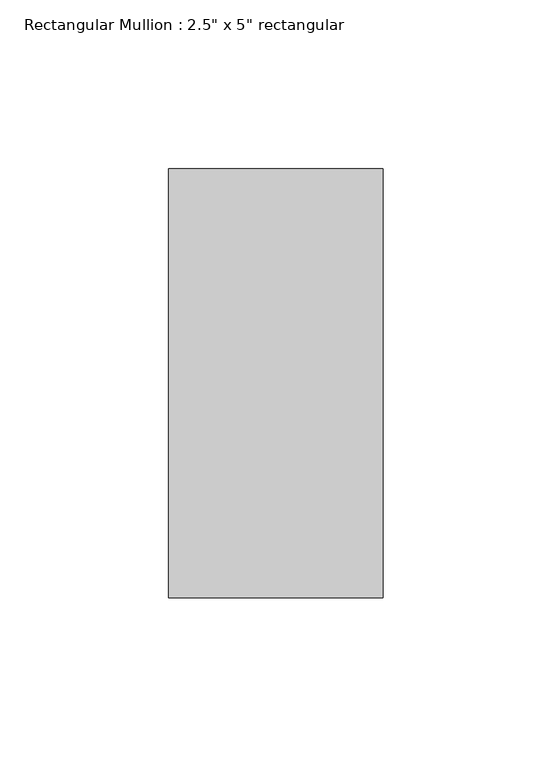
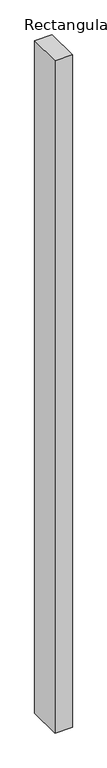
"""IFC4 building model written with IfcOpenShell, lengths in millimetres: member geometry."""

from ifc_helpers import new_model, si_unit, frame, origin, place, context, project, spatial, polyline, outline, extrude, source, transform, mapped, element, save


def member_bee07d73(model_context):
    return source(origin(), model_context, "Body", "SweptSolid", [
        extrude(outline(polyline([(0.0, 63.5), (0.0, -63.5), (-63.5, -63.5), (-63.5, 63.5), (0.0, 63.5)])), frame((0.0, 0.0, -2581.7369027), z_axis=(0.0, 0.0, 1.0), x_axis=(1.0, 0.0, 0.0)), (0.0, 0.0, 1.0), 2581.7369027),
    ])


if __name__ == "__main__":
    model = new_model("IFC4")
    model_context = context("Model", 3, world=origin())
    ifc_project = project(units=[si_unit("LENGTHUNIT", "METRE", prefix="MILLI")], contexts=[model_context])
    site = spatial("IfcSite", under=ifc_project)
    building = spatial("IfcBuilding", under=site)
    placement = place(None, origin())
    member_shape = member_bee07d73(model_context)
    element("IfcMember", 1, ObjectType="Rectangular Mullion : 2.5\" x 5\" rectangular", at=placement, inside=building, context=model_context, shape_type="MappedRepresentation", body=[
        mapped(member_shape, transform((0.0, 0.0, 0.0), x_axis=(1.0, 0.0, 0.0), y_axis=(0.0, 1.0, 0.0), z_axis=(0.0, 0.0, 1.0))),
    ])
    save(model, "model.ifc")

# Revit data of these elements
# Type "Rectangular Mullion : 2.5\" x 5\" rectangular"
#   built-in parameter 1007304 = 0.416667 (stored number, unit not read)
#   built-in parameter 1007301 = 0.104167 (stored number, unit not read)
#   built-in parameter 1007300 = 0.104167 (stored number, unit not read)
# Element 1 (IfcMember, "Rectangular Mullion : 2.5\" x 5\" rectangular")
#   Materials on its faces: "Gypsum Wall Board"
# Materials
#   "Gypsum Wall Board": class "Generic", colour RGB 127 127 127, transparency 0, Description = "Gypsum Wall Board", Cost = 0
